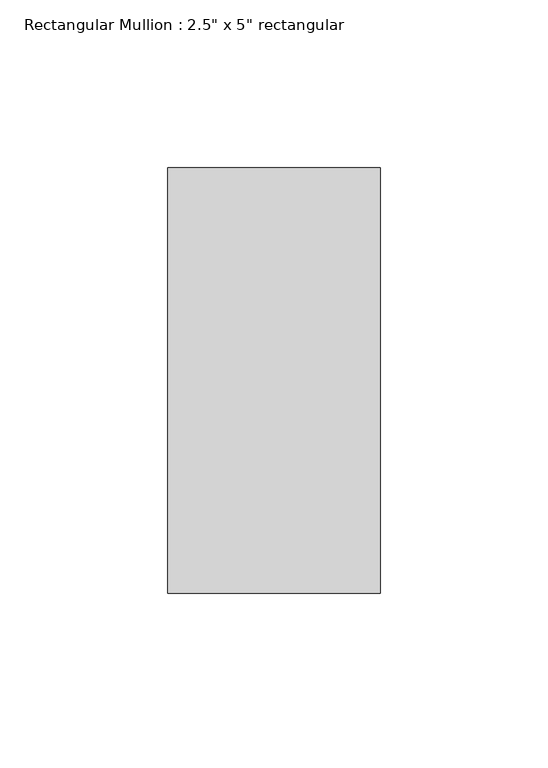
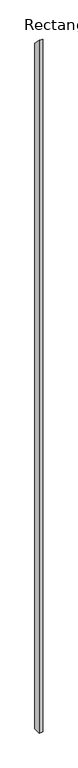
"""IFC4 building model written with IfcOpenShell, lengths in millimetres: member geometry."""

from ifc_helpers import new_model, si_unit, frame, origin, place, context, project, spatial, polyline, outline, extrude, source, transform, mapped, element, save


def member_b1296a21(model_context):
    return source(origin(), model_context, "Body", "SweptSolid", [
        extrude(outline(polyline([(-63.5, 63.5), (63.5, -63.5), (63.5, -12700.2660719), (-63.5, -12700.2660719), (-63.5, 63.5)])), frame((-63.5, 0.0, 0.0), z_axis=(1.0, 0.0, 0.0), x_axis=(0.0, 1.0, 0.0)), (0.0, 0.0, 1.0), 63.5),
    ])


if __name__ == "__main__":
    model = new_model("IFC4")
    model_context = context("Model", 3, world=origin())
    ifc_project = project(units=[si_unit("LENGTHUNIT", "METRE", prefix="MILLI")], contexts=[model_context])
    site = spatial("IfcSite", under=ifc_project)
    building = spatial("IfcBuilding", under=site)
    placement = place(None, origin())
    member_shape = member_b1296a21(model_context)
    element("IfcMember", 1, ObjectType="Rectangular Mullion : 2.5\" x 5\" rectangular", at=placement, inside=building, context=model_context, shape_type="MappedRepresentation", body=[
        mapped(member_shape, transform((0.0, 0.0, 0.0), x_axis=(1.0, 0.0, 0.0), y_axis=(0.0, 1.0, 0.0), z_axis=(0.0, 0.0, 1.0))),
    ])
    save(model, "model.ifc")

# Revit data of these elements
# Type "Rectangular Mullion : 2.5\" x 5\" rectangular"
#   built-in parameter 1007304 = 0.416667 (stored number, unit not read)
#   built-in parameter 1007301 = 0.104167 (stored number, unit not read)
#   built-in parameter 1007300 = 0.104167 (stored number, unit not read)
# Element 1 (IfcMember, "Rectangular Mullion : 2.5\" x 5\" rectangular")
#   Materials on its faces: "Aluminum"
# Materials
#   "Aluminum": class "Metal", colour RGB 247 247 247, transparency 0, Description = "Aluminum 6061", Cost = 0
